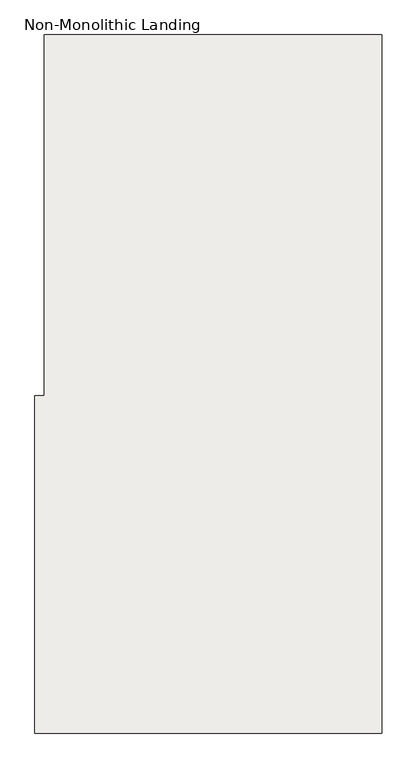
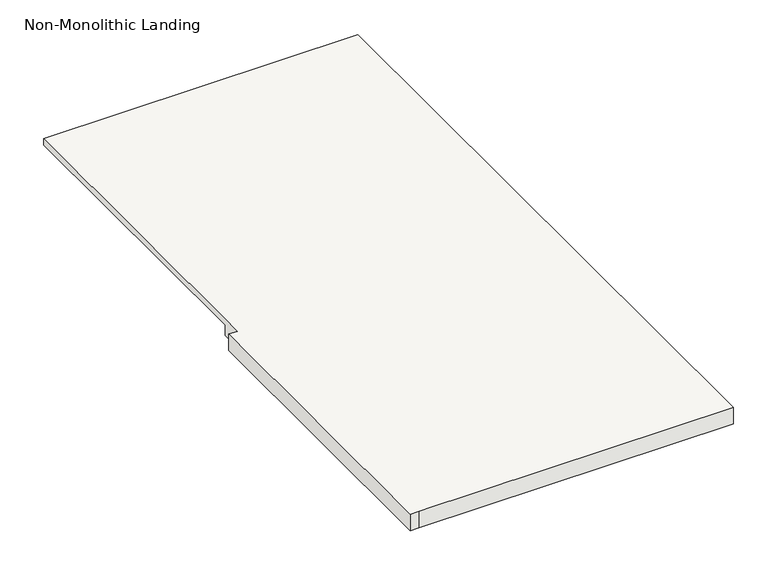
"""IFC4 building model written with IfcOpenShell, lengths in millimetres: slab geometry, Non-Monolithic Landing."""

from ifc_helpers import new_model, si_unit, origin, place, context, project, spatial, faceted_brep, source, transform, mapped, element, save


def non_monolithic_landing_275f9134(model_context):
    return source(origin(), model_context, "Body", "Brep", [
        faceted_brep([(-1690.2851125, 2156.5395264, 1504.95), (-1664.8851125, 2156.5395264, 1479.55), (-1664.8851125, 1242.1395264, 1479.55), (-1690.2851125, 1242.1395264, 1504.95), (-1690.2851125, 1179.1428815, 1524.0), (-1715.6851125, 1179.1428815, 1524.0), (-1715.6851125, 264.7428815, 1524.0), (-1690.2851125, 264.7428815, 1524.0), (-775.8851125, 264.7428815, 1524.0), (-775.8851125, 2156.5395264, 1524.0), (-1690.2851125, 2156.5395264, 1524.0), (-1664.8851125, 1242.1395264, 1473.2), (-1664.8851125, 2156.5395264, 1473.2), (-775.8851125, 2156.5395264, 1473.2), (-775.8851125, 264.7428815, 1473.2), (-1690.2851125, 264.7428815, 1473.2), (-1715.6851125, 264.7428815, 1473.2), (-1715.6851125, 1179.1428815, 1473.2), (-1690.2851125, 1179.1428815, 1473.2), (-1690.2851125, 1242.1395264, 1473.2)], [[[0, 1, 2, 3]], [[4, 5, 6, 7, 8, 9, 10]], [[11, 12, 13, 14, 15, 16, 17, 18, 19]], [[12, 11, 2, 1]], [[11, 19, 3, 2]], [[4, 10, 0, 3, 19, 18]], [[5, 4, 18, 17]], [[6, 5, 17, 16]], [[7, 6, 16, 15]], [[8, 7, 15, 14]], [[9, 8, 14, 13]], [[10, 9, 13, 12, 1, 0]]]),
    ])


if __name__ == "__main__":
    model = new_model("IFC4")
    model_context = context("Model", 3, world=origin())
    ifc_project = project(units=[si_unit("LENGTHUNIT", "METRE", prefix="MILLI")], contexts=[model_context])
    site = spatial("IfcSite", under=ifc_project)
    building = spatial("IfcBuilding", under=site)
    placement = place(None, origin())
    non_monolithic_landing_shape = non_monolithic_landing_275f9134(model_context)
    element("IfcSlab", 1, ObjectType="Non-Monolithic Landing", at=placement, inside=building, context=model_context, shape_type="MappedRepresentation", body=[
        mapped(non_monolithic_landing_shape, transform((0.0, 0.0, 0.0), x_axis=(1.0, 0.0, 0.0), y_axis=(0.0, 1.0, 0.0), z_axis=(0.0, 0.0, 1.0))),
    ])
    save(model, "model.ifc")
